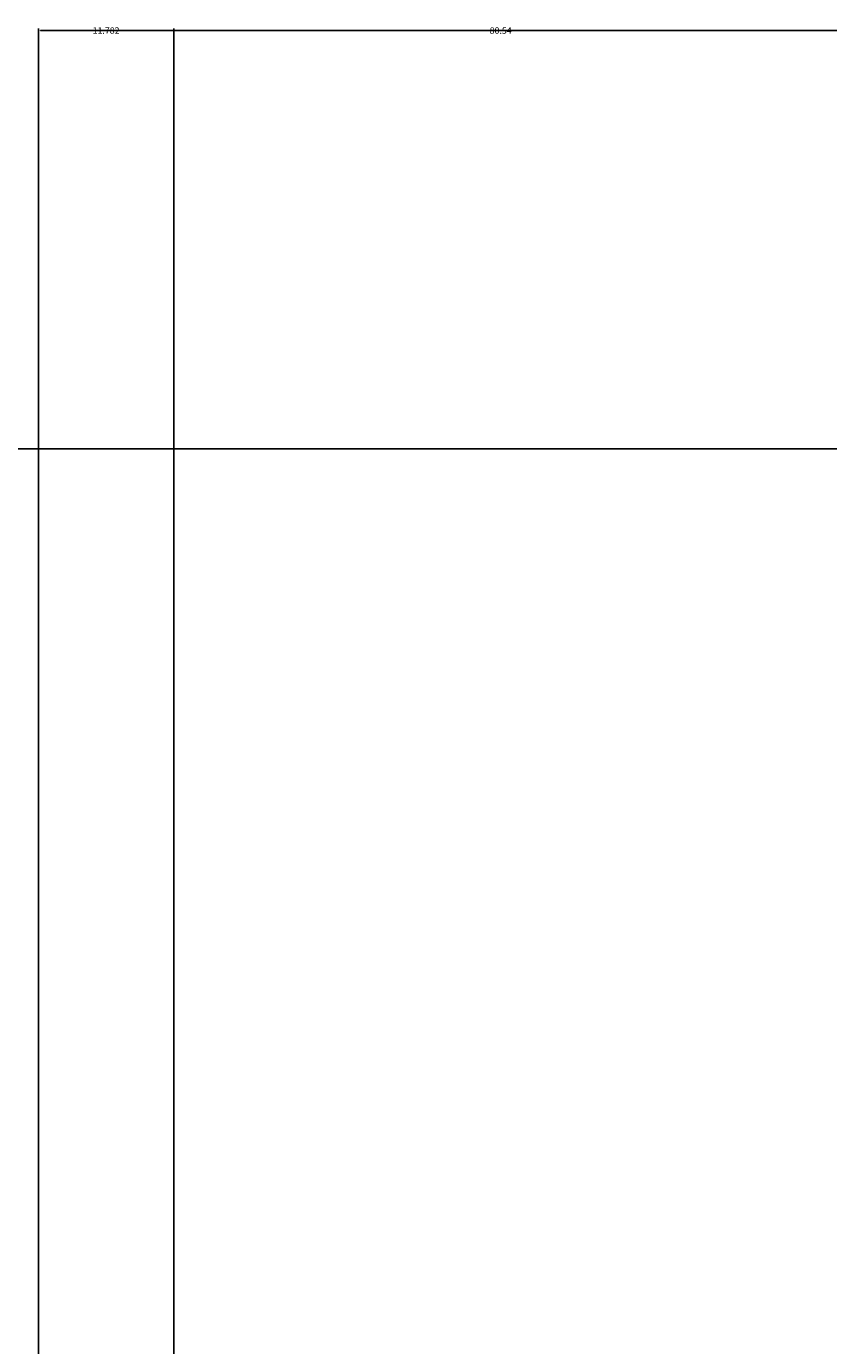
# Model space of a CAD drawing. Units: inches. Extents: x -26 to 776, y -22 to 650.
# Tile 30 of 62: x 10 to 80, y 535 to 650. Entities that reach past the tile are written whole.
import ezdxf

# ---------------------------------------------------------------- set-up
doc = ezdxf.new("R2010")
doc.units = ezdxf.units.IN
doc.header["$MEASUREMENT"] = 0
doc.layers.add('A-ANNO-DIMS', color=2, linetype='Continuous', lineweight=18)
doc.styles.get("Standard").update_dxf_attribs({"font": 'arial.ttf'})
doc.dimstyles.get("Standard").update_dxf_attribs({"dimtxt": 0.5625, "dimasz": 0.18, "dimexe": 0.18, "dimexo": 0.0625, "dimgap": 0.09, "dimtad": 0, "dimtih": 1, "dimtoh": 1, "dimdec": 4, "dimzin": 0, "dimdsep": 46, "dimlunit": 4, "dimtxsty": 'Standard', "dimcen": 0.09, "dimadec": 0, "dimazin": 0, "dimtfac": 1, "dimtdec": 4, "dimtofl": 0, "dimtmove": 0, "dimatfit": 3, "dimfxl": 1, "dimtolj": 1, "dimtzin": 0, "dimarcsym": 0})

# ---------------------------------------------------------------- blocks, each defined once
blk = doc.blocks.new('*D14')
at = {"layer": 'A-ANNO-DIMS', "color": 0, "lineweight": -2, "transparency": 16777216}
for p, q in [((191.62, 613.27), (-25.48, 613.27)), ((-25.3, 613.09), (-25.3, 314.75)), ((-25.3, 15.66), (-25.3, 314)), ((11.04, 15.48), (-25.48, 15.48))]:
    blk.add_line(p, q, dxfattribs=at)
at = {"layer": 'A-ANNO-DIMS', "color": 0, "transparency": 16777216}
for points in [[(-25.33, 613.09), (-25.27, 613.09), (-25.3, 613.27)], [(-25.33, 15.66), (-25.27, 15.66), (-25.3, 15.48)]]:
    blk.add_solid(points, dxfattribs=at)
at = {"layer": 'Defpoints', "color": 0, "transparency": 16777216}
for p in [(-25.3, 613.27), (191.68, 613.27), (11.11, 15.48)]:
    blk.add_point(p, dxfattribs=at)
at = {"layer": 'A-ANNO-DIMS', "color": 0, "transparency": 16777216, "insert": (-25.3, 314.38), "char_height": 0.562, "attachment_point": 5}
blk.add_mtext('\\A1;597.8', dxfattribs=at)
blk = doc.blocks.new('*D15')
at = {"layer": 'A-ANNO-DIMS', "color": 0, "lineweight": -2, "transparency": 16777216}
for p, q in [((11.11, 491.49), (11.11, 649.86)), ((11.29, 649.68), (120.22, 649.68)), ((231.24, 649.68), (122.31, 649.68)), ((231.42, 491.49), (231.42, 649.86))]:
    blk.add_line(p, q, dxfattribs=at)
at = {"layer": 'A-ANNO-DIMS', "color": 0, "transparency": 16777216}
for points in [[(11.29, 649.71), (11.29, 649.65), (11.11, 649.68)], [(231.24, 649.71), (231.24, 649.65), (231.42, 649.68)]]:
    blk.add_solid(points, dxfattribs=at)
at = {"layer": 'Defpoints', "color": 0, "transparency": 16777216}
for p in [(231.42, 649.68), (11.11, 491.43), (231.42, 491.43)]:
    blk.add_point(p, dxfattribs=at)
at = {"layer": 'A-ANNO-DIMS', "color": 0, "transparency": 16777216, "insert": (121.27, 649.68), "char_height": 0.562, "attachment_point": 5}
blk.add_mtext('\\A1;220.3', dxfattribs=at)
blk = doc.blocks.new('*D17')
at = {"layer": 'A-ANNO-DIMS', "color": 0, "lineweight": -2, "transparency": 16777216}
for p, q in [((11.11, 491.49), (11.11, 649.86)), ((11.29, 649.68), (100.16, 649.68)), ((191.5, 649.68), (102.62, 649.68)), ((191.68, 613.33), (191.68, 649.86))]:
    blk.add_line(p, q, dxfattribs=at)
at = {"layer": 'A-ANNO-DIMS', "color": 0, "transparency": 16777216}
for points in [[(11.29, 649.71), (11.29, 649.65), (11.11, 649.68)], [(191.5, 649.71), (191.5, 649.65), (191.68, 649.68)]]:
    blk.add_solid(points, dxfattribs=at)
at = {"layer": 'Defpoints', "color": 0, "transparency": 16777216}
for p in [(191.68, 649.68), (191.68, 613.27), (11.11, 491.43)]:
    blk.add_point(p, dxfattribs=at)
at = {"layer": 'A-ANNO-DIMS', "color": 0, "transparency": 16777216, "insert": (101.39, 649.68), "char_height": 0.562, "attachment_point": 5}
blk.add_mtext('\\A1;180.57', dxfattribs=at)
blk = doc.blocks.new('*D19')
at = {"layer": 'A-ANNO-DIMS', "color": 0, "lineweight": -2, "transparency": 16777216}
for p, q in [((191.62, 613.27), (-25.48, 613.27)), ((-25.3, 613.09), (-25.3, 552.73)), ((-25.3, 491.61), (-25.3, 551.97)), ((191.62, 491.43), (-25.48, 491.43))]:
    blk.add_line(p, q, dxfattribs=at)
at = {"layer": 'A-ANNO-DIMS', "color": 0, "transparency": 16777216}
for points in [[(-25.33, 613.09), (-25.27, 613.09), (-25.3, 613.27)], [(-25.33, 491.61), (-25.27, 491.61), (-25.3, 491.43)]]:
    blk.add_solid(points, dxfattribs=at)
at = {"layer": 'Defpoints', "color": 0, "transparency": 16777216}
for p in [(-25.3, 613.27), (191.68, 613.27), (191.68, 491.43)]:
    blk.add_point(p, dxfattribs=at)
at = {"layer": 'A-ANNO-DIMS', "color": 0, "transparency": 16777216, "insert": (-25.3, 552.35), "char_height": 0.562, "attachment_point": 5}
blk.add_mtext('\\A1;121.84', dxfattribs=at)
blk = doc.blocks.new('*D22')
at = {"layer": 'A-ANNO-DIMS', "color": 0, "lineweight": -2, "transparency": 16777216}
for p, q in [((22.89, 15.33), (22.89, 649.86)), ((23.07, 649.68), (119.19, 649.68)), ((217.77, 649.68), (121.65, 649.68)), ((217.95, 15.54), (217.95, 649.86))]:
    blk.add_line(p, q, dxfattribs=at)
at = {"layer": 'A-ANNO-DIMS', "color": 0, "transparency": 16777216}
for points in [[(23.07, 649.71), (23.07, 649.65), (22.89, 649.68)], [(217.77, 649.71), (217.77, 649.65), (217.95, 649.68)]]:
    blk.add_solid(points, dxfattribs=at)
at = {"layer": 'Defpoints', "color": 0, "transparency": 16777216}
for p in [(217.95, 649.68), (22.89, 15.27), (217.95, 15.48)]:
    blk.add_point(p, dxfattribs=at)
at = {"layer": 'A-ANNO-DIMS', "color": 0, "transparency": 16777216, "insert": (120.42, 649.68), "char_height": 0.562, "attachment_point": 5}
blk.add_mtext('\\A1;195.06', dxfattribs=at)
blk = doc.blocks.new('*D24')
at = {"layer": 'A-ANNO-DIMS', "color": 0, "lineweight": -2, "transparency": 16777216}
for p, q in [((11.11, 15.54), (11.11, 649.86)), ((11.29, 649.68), (15.77, 649.68)), ((22.71, 649.68), (18.23, 649.68)), ((22.89, 15.33), (22.89, 649.86))]:
    blk.add_line(p, q, dxfattribs=at)
at = {"layer": 'A-ANNO-DIMS', "color": 0, "transparency": 16777216}
for points in [[(11.29, 649.71), (11.29, 649.65), (11.11, 649.68)], [(22.71, 649.71), (22.71, 649.65), (22.89, 649.68)]]:
    blk.add_solid(points, dxfattribs=at)
at = {"layer": 'Defpoints', "color": 0, "transparency": 16777216}
for p in [(22.89, 649.68), (11.11, 15.48), (22.89, 15.27)]:
    blk.add_point(p, dxfattribs=at)
at = {"layer": 'A-ANNO-DIMS', "color": 0, "transparency": 16777216, "insert": (17, 649.68), "char_height": 0.562, "attachment_point": 5}
blk.add_mtext('\\A1;11.782', dxfattribs=at)
blk = doc.blocks.new('*D25')
at = {"layer": 'A-ANNO-DIMS', "color": 0, "lineweight": -2, "transparency": 16777216}
for p, q in [((11.11, 221.7), (11.11, 649.86)), ((11.29, 649.68), (50.34, 649.68)), ((91.46, 649.68), (52.41, 649.68)), ((91.64, 271.37), (91.64, 649.86))]:
    blk.add_line(p, q, dxfattribs=at)
at = {"layer": 'A-ANNO-DIMS', "color": 0, "transparency": 16777216}
for points in [[(11.29, 649.71), (11.29, 649.65), (11.11, 649.68)], [(91.46, 649.71), (91.46, 649.65), (91.64, 649.68)]]:
    blk.add_solid(points, dxfattribs=at)
at = {"layer": 'Defpoints', "color": 0, "transparency": 16777216}
for p in [(91.64, 649.68), (91.64, 271.31), (11.11, 221.64)]:
    blk.add_point(p, dxfattribs=at)
at = {"layer": 'A-ANNO-DIMS', "color": 0, "transparency": 16777216, "insert": (51.38, 649.68), "char_height": 0.562, "attachment_point": 5}
blk.add_mtext('\\A1;80.54', dxfattribs=at)

msp = doc.modelspace()

# ---------------------------------------------------------------- dimensions: what is measured, and where the dimension line sits
at = {"layer": 'A-ANNO-DIMS'}
for base, p1, p2, override, picture, middle in [((231.4249, 649.6763), (11.1074, 491.4269), (231.4249, 491.4269), {"dimdec": 1, "dimlfac": 1, "dimrnd": 0, "dimzin": 0, "dimdsep": 46, "dimlunit": 2}, '*D15', (121.2661, 649.6763)), ((191.6782, 649.6763), (11.1074, 491.4269), (191.6782, 613.2713), {"dimdec": 2, "dimlfac": 1, "dimrnd": 0, "dimzin": 0, "dimdsep": 46, "dimlunit": 2}, '*D17', (101.3928, 649.6763)), ((22.8891, 649.6763), (11.1074, 15.4824), (22.8891, 15.2701), {"dimdec": 3, "dimlfac": 1, "dimrnd": 0, "dimzin": 0, "dimdsep": 46, "dimlunit": 2}, '*D24', (16.9982, 649.6763)), ((91.6448, 649.6763), (11.1074, 221.6413), (91.6448, 271.3091), {"dimdec": 2, "dimlfac": 1, "dimrnd": 0, "dimzin": 0, "dimdsep": 46, "dimlunit": 2}, '*D25', (51.3761, 649.6763)), ((217.9529, 649.6763), (22.8891, 15.2701), (217.9529, 15.4824), {"dimdec": 2, "dimlfac": 1, "dimrnd": 0, "dimzin": 0, "dimdsep": 46, "dimlunit": 2}, '*D22', (120.421, 649.6763))]:
    dim = msp.add_linear_dim(base=base, p1=p1, p2=p2, dimstyle='Standard', override=override, dxfattribs=at)
    dim.commit()
    dim.dimension.update_dxf_attribs({"geometry": picture, "text_midpoint": middle})
for p1, override, picture, middle in [((191.6782, 491.4269), {"dimdec": 2, "dimlfac": 1, "dimrnd": 0, "dimzin": 0, "dimdsep": 46, "dimlunit": 2}, '*D19', (-25.2976, 552.3491)), ((11.1074, 15.4824), {"dimdec": 1, "dimlfac": 1, "dimrnd": 0, "dimzin": 0, "dimdsep": 46, "dimlunit": 2}, '*D14', (-25.2976, 314.3769))]:
    dim = msp.add_linear_dim(base=(-25.2976, 613.2713), p1=p1, p2=(191.6782, 613.2713), angle=90, dimstyle='Standard', override=override, dxfattribs=at)
    dim.commit()
    dim.dimension.update_dxf_attribs({"geometry": picture, "text_midpoint": middle})

doc.saveas('drawing.dxf')
